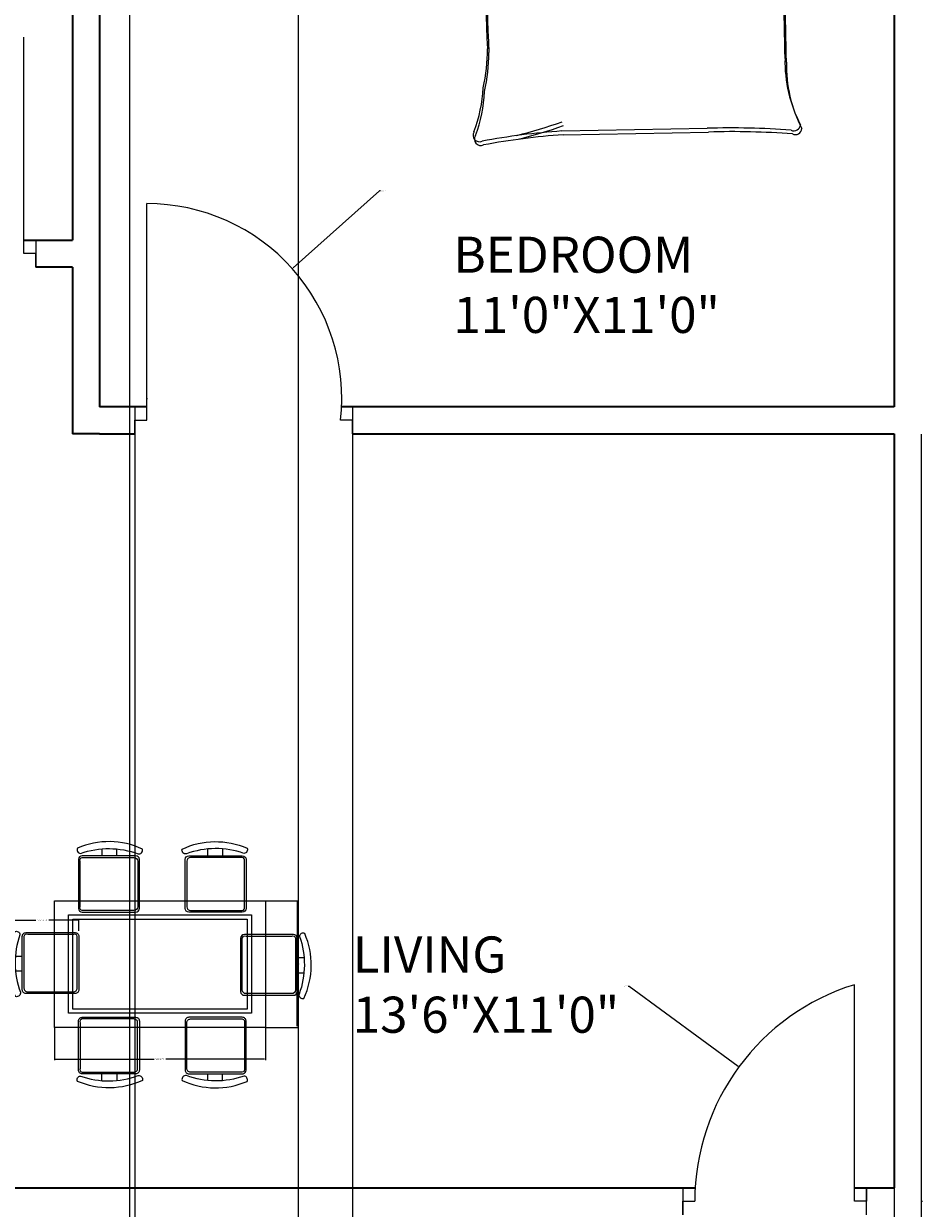
# Model space of a CAD drawing. Units: inches. Extents: x 1721 to 2510, y 1544 to 2360.
# Tile 7 of 10: x 1940 to 2090, y 1988 to 2185. Entities that reach past the tile are written whole.
import ezdxf

# ---------------------------------------------------------------- set-up
doc = ezdxf.new("R2010")
doc.units = ezdxf.units.IN
for name, color, linetype, lineweight in [('A-ANNO-DIMS', 2, 'Continuous', 18), ('A-AREA-IDEN', 7, 'Continuous', 18), ('A-DOOR', 3, 'Continuous', 18), ('A-FURN', 8, 'Continuous', 13), ('A-WALL', 7, 'Continuous', 35)]:
    doc.layers.add(name, color=color, linetype=linetype, lineweight=lineweight)
doc.styles.get("Standard").update_dxf_attribs({"font": 'arial.ttf'})
doc.dimstyles.get("Standard").update_dxf_attribs({"dimtxt": 0.18, "dimasz": 0.18, "dimexe": 0.18, "dimexo": 0.0625, "dimgap": 0.09, "dimtad": 0, "dimtih": 1, "dimtoh": 1, "dimdec": 4, "dimzin": 0, "dimdsep": 46, "dimtxsty": 'Standard', "dimcen": 0.09, "dimadec": 0, "dimazin": 0, "dimtfac": 1, "dimtdec": 4, "dimtofl": 0, "dimtmove": 0, "dimatfit": 3, "dimfxl": 1, "dimtolj": 1, "dimtzin": 0, "dimarcsym": 0})

# ---------------------------------------------------------------- blocks, each defined once
blk = doc.blocks.new('BED-DOUBLE')
for p, q in [((39.64, 78.43), (15.52, 78.72)), ((39.64, 78.43), (15.52, 78.72)), ((39.86, 77.8), (15.74, 78.09)), ((39.86, 77.8), (15.74, 78.09)), ((1.93, 30.11), (1.99, 28.4, 3.79)), ((1.93, 30.11), (1.99, 28.4, 3.79)), ((15.66, 30.21), (13.68, 29.32)), ((15.66, 30.21), (13.68, 29.32)), ((15.88, 29.58), (13.89, 28.69)), ((15.88, 29.58), (13.89, 28.69)), ((18.1, 30.79), (15.66, 30.21)), ((18.1, 30.79), (15.66, 30.21)), ((18.31, 30.16), (15.88, 29.58)), ((18.31, 30.16), (15.88, 29.58)), ((18.38, 28.81), (18.1, 30.79)), ((18.38, 28.81), (18.1, 30.79)), ((18.59, 28.18), (18.31, 30.16)), ((18.59, 28.18), (18.31, 30.16)), ((3.5, 28.99), (1.99, 28.4)), ((3.5, 28.99), (1.99, 28.4)), ((1.99, 28.4), (5.58, 25.17)), ((1.99, 28.4), (5.58, 25.17)), ((2.15, 29.48), (2.21, 27.77, 3.79)), ((2.15, 29.48), (2.21, 27.77, 3.79)), ((3.72, 28.36), (2.21, 27.77)), ((3.72, 28.36), (2.21, 27.77)), ((2.21, 27.77), (5.8, 24.54)), ((2.21, 27.77), (5.8, 24.54)), ((6.54, 28.65), (3.5, 28.99)), ((6.54, 28.65), (3.5, 28.99)), ((6.75, 28.02), (3.72, 28.36)), ((6.75, 28.02), (3.72, 28.36)), ((10.33, 28.91), (6.54, 28.65)), ((10.33, 28.91), (6.54, 28.65)), ((10.55, 28.28), (6.75, 28.02)), ((10.55, 28.28), (6.75, 28.02)), ((13.68, 29.32), (10.33, 28.91)), ((13.68, 29.32), (10.33, 28.91)), ((13.89, 28.69), (10.55, 28.28)), ((13.89, 28.69), (10.55, 28.28)), ((20, 24.39), (18.38, 28.81)), ((20, 24.39), (18.38, 28.81)), ((20.21, 23.76), (18.59, 28.18)), ((20.21, 23.76), (18.59, 28.18)), ((3.23, 1.19), (3.55, 27.27)), ((3.23, 1.19), (3.55, 27.27)), ((3.45, 0.56), (3.76, 26.64)), ((3.45, 0.56), (3.76, 26.64)), ((5.58, 25.17), (8.44, 23.01)), ((5.58, 25.17), (8.44, 23.01)), ((5.8, 24.54), (8.66, 22.38)), ((5.8, 24.54), (8.66, 22.38)), ((24.03, 17.98), (20, 24.39)), ((24.03, 17.98), (20, 24.39)), ((24.24, 17.35), (20.21, 23.76)), ((24.24, 17.35), (20.21, 23.76)), ((8.44, 23.01), (13.88, 20.98)), ((8.44, 23.01), (13.88, 20.98)), ((8.66, 22.38), (14.1, 20.35)), ((8.66, 22.38), (14.1, 20.35)), ((13.88, 20.98), (22.02, 18)), ((13.88, 20.98), (22.02, 18)), ((14.1, 20.35), (22.24, 17.37)), ((14.1, 20.35), (22.24, 17.37)), ((50.28, 18.38), (50.07, 0.63)), ((50.28, 18.38), (50.07, 0.63)), ((50.5, 17.75), (50.29, 0)), ((50.5, 17.75), (50.29, 0)), ((9.01, 16.97), (3.98, 17.42)), ((3.98, 17.42), (4.71, 14.34)), ((9.01, 16.97), (3.98, 17.42)), ((3.98, 17.42), (4.71, 14.34)), ((9.23, 16.34), (4.2, 16.8)), ((4.2, 16.8), (4.92, 13.71)), ((9.23, 16.34), (4.2, 16.8)), ((4.2, 16.8), (4.92, 13.71)), ((10.94, 17.49), (9.01, 16.97)), ((10.94, 17.49), (9.01, 16.97)), ((11.15, 16.86), (9.23, 16.34)), ((11.15, 16.86), (9.23, 16.34)), ((17.8, 16.99), (10.94, 17.49)), ((17.8, 16.99), (10.94, 17.49)), ((18.02, 16.36), (11.15, 16.86)), ((18.02, 16.36), (11.15, 16.86)), ((21.75, 16.29), (17.8, 16.99)), ((21.75, 16.29), (17.8, 16.99)), ((21.96, 15.66), (18.02, 16.36)), ((21.96, 15.66), (18.02, 16.36)), ((23.54, 17.35), (20.51, 16.13)), ((23.54, 17.35), (20.51, 16.13)), ((23.75, 16.73), (20.73, 15.5)), ((23.75, 16.73), (20.73, 15.5)), ((25.94, 17.48), (23.54, 17.35)), ((25.94, 17.48), (23.54, 17.35)), ((26.16, 16.85), (23.75, 16.73)), ((26.16, 16.85), (23.75, 16.73)), ((26.07, 14.85), (25.94, 17.48)), ((26.07, 14.85), (25.94, 17.48)), ((26.29, 14.22), (26.16, 16.85)), ((26.29, 14.22), (26.16, 16.85)), ((27.61, 14.21), (27.64, 16.84)), ((27.61, 14.21), (27.64, 16.84)), ((27.64, 16.84), (30.05, 16.81)), ((27.64, 16.84), (30.05, 16.81)), ((27.82, 13.58), (27.85, 16.21)), ((27.82, 13.58), (27.85, 16.21)), ((27.85, 16.21), (30.26, 16.18)), ((27.85, 16.21), (30.26, 16.18)), ((34.67, 16.66), (29.65, 17.12)), ((34.67, 16.66), (29.65, 17.12)), ((34.89, 16.03), (29.86, 16.49)), ((34.89, 16.03), (29.86, 16.49)), ((30.05, 16.81), (33.11, 15.7)), ((30.05, 16.81), (33.11, 15.7)), ((30.26, 16.18), (33.33, 15.07)), ((30.26, 16.18), (33.33, 15.07)), ((36.6, 17.19), (34.67, 16.66)), ((36.6, 17.19), (34.67, 16.66)), ((36.81, 16.56), (34.89, 16.03)), ((36.81, 16.56), (34.89, 16.03)), ((43.46, 16.68), (36.6, 17.19)), ((43.46, 16.68), (36.6, 17.19)), ((43.68, 16.05), (36.81, 16.56)), ((43.68, 16.05), (36.81, 16.56)), ((43.46, 16.68), (44.58, 16.98)), ((43.46, 16.68), (44.58, 16.98)), ((47.41, 15.98), (43.46, 16.68)), ((47.41, 15.98), (43.46, 16.68)), ((43.68, 16.05), (44.79, 16.35)), ((43.68, 16.05), (44.79, 16.35)), ((47.62, 15.35), (43.68, 16.05)), ((47.62, 15.35), (43.68, 16.05)), ((44.58, 16.98), (49.58, 17.63)), ((44.58, 16.98), (49.58, 17.63)), ((44.79, 16.35), (49.8, 17)), ((44.79, 16.35), (49.8, 17)), ((49.58, 17.63), (48.98, 14.52)), ((49.58, 17.63), (48.98, 14.52)), ((49.8, 17), (49.19, 13.89)), ((49.8, 17), (49.19, 13.89)), ((4.71, 14.34), (4.5, 12.77)), ((4.71, 14.34), (4.5, 12.77)), ((26.73, 13.04), (26.07, 14.85)), ((26.73, 13.04), (26.07, 14.85)), ((26.95, 12.41), (26.29, 14.22)), ((26.95, 12.41), (26.29, 14.22)), ((27.02, 12.38), (27.61, 14.21)), ((27.02, 12.38), (27.61, 14.21)), ((48.98, 14.52), (49.24, 12.96)), ((48.98, 14.52), (49.24, 12.96)), ((49.19, 13.89), (49.46, 12.33)), ((49.19, 13.89), (49.46, 12.33)), ((4.5, 12.77), (5.25, 9.26)), ((4.5, 12.77), (5.25, 9.26)), ((4.92, 13.71), (4.72, 12.14)), ((4.92, 13.71), (4.72, 12.14)), ((4.72, 12.14), (5.46, 8.63)), ((4.72, 12.14), (5.46, 8.63)), ((26.8, 11.77), (26.73, 13.04)), ((26.8, 11.77), (26.73, 13.04)), ((27.01, 11.14), (26.95, 12.41)), ((27.01, 11.14), (26.95, 12.41)), ((27, 11.1), (27.02, 12.38)), ((27, 11.1), (27.02, 12.38)), ((27.23, 11.75), (27.82, 13.58)), ((27.23, 11.75), (27.82, 13.58)), ((49.24, 12.96), (48.63, 9.42)), ((49.24, 12.96), (48.63, 9.42)), ((49.46, 12.33), (48.85, 8.79)), ((49.46, 12.33), (48.85, 8.79)), ((4.25, 9.35), (4.77, 10.37)), ((4.25, 9.35), (4.77, 10.37)), ((26.39, 8.62), (26.8, 11.77)), ((26.39, 8.62), (26.8, 11.77)), ((26.61, 7.99), (27.01, 11.14)), ((26.61, 7.99), (27.01, 11.14)), ((27.53, 7.98), (27, 11.1)), ((27.53, 7.98), (27, 11.1)), ((27.22, 10.47), (27.23, 11.75)), ((27.22, 10.47), (27.23, 11.75)), ((27.75, 7.35), (27.22, 10.47)), ((27.75, 7.35), (27.22, 10.47)), ((49.63, 9.55), (49.07, 10.55)), ((49.63, 9.55), (49.07, 10.55)), ((49.84, 8.92), (49.29, 9.92)), ((49.84, 8.92), (49.29, 9.92)), ((4.8, 6.82), (4.25, 9.35)), ((4.8, 6.82), (4.25, 9.35)), ((4.47, 8.72), (4.98, 9.74)), ((4.47, 8.72), (4.98, 9.74)), ((5.02, 6.19), (4.47, 8.72)), ((5.02, 6.19), (4.47, 8.72)), ((5.25, 9.26), (6.37, 6.62)), ((5.25, 9.26), (6.37, 6.62)), ((5.46, 8.63), (6.59, 5.99)), ((5.46, 8.63), (6.59, 5.99)), ((26.09, 3.36), (26.39, 8.62)), ((26.09, 3.36), (26.39, 8.62)), ((26.3, 2.73), (26.61, 7.99)), ((26.3, 2.73), (26.61, 7.99)), ((28.04, 2.73), (27.53, 7.98)), ((28.04, 2.73), (27.53, 7.98)), ((48.63, 9.42), (47.61, 6.74)), ((48.63, 9.42), (47.61, 6.74)), ((48.85, 8.79), (47.82, 6.11)), ((48.85, 8.79), (47.82, 6.11)), ((49.17, 7.01), (49.63, 9.55)), ((49.17, 7.01), (49.63, 9.55)), ((49.39, 6.38), (49.84, 8.92)), ((49.39, 6.38), (49.84, 8.92)), ((4.39, 3.68), (4.8, 6.82)), ((4.39, 3.68), (4.8, 6.82)), ((4.61, 3.05), (5.02, 6.19)), ((4.61, 3.05), (5.02, 6.19)), ((28.25, 2.1), (27.75, 7.35)), ((28.25, 2.1), (27.75, 7.35)), ((49.7, 3.88), (49.17, 7.01)), ((49.7, 3.88), (49.17, 7.01)), ((49.92, 3.25), (49.39, 6.38)), ((49.92, 3.25), (49.39, 6.38)), ((8.71, 3.62), (12.44, 4.09)), ((8.71, 3.62), (12.44, 4.09)), ((12.44, 4.09), (17.76, 5.35)), ((12.44, 4.09), (17.76, 5.35)), ((12.65, 3.46), (17.98, 4.72)), ((12.65, 3.46), (17.98, 4.72)), ((15.1, 4.65), (17.12, 4.04)), ((15.1, 4.65), (17.12, 4.04)), ((15.32, 4.02), (17.34, 3.41)), ((15.32, 4.02), (17.34, 3.41)), ((17.12, 4.04), (19.98, 3.48)), ((17.12, 4.04), (19.98, 3.48)), ((41.65, 3.98), (36.28, 5.04)), ((41.65, 3.98), (36.28, 5.04)), ((41.87, 3.35), (36.49, 4.41)), ((41.87, 3.35), (36.49, 4.41)), ((38.96, 4.44), (36.97, 3.75)), ((38.96, 4.44), (36.97, 3.75)), ((45.39, 3.65), (41.65, 3.98)), ((45.39, 3.65), (41.65, 3.98)), ((50.09, 2.13), (3.25, 2.69)), ((50.09, 2.13), (3.25, 2.69)), ((50.31, 1.5), (3.47, 2.06)), ((50.31, 1.5), (3.47, 2.06)), ((4.39, 3.68), (9.69, 3.52)), ((4.39, 3.68), (9.69, 3.52)), ((4.61, 3.05), (9.9, 2.89)), ((4.61, 3.05), (9.9, 2.89)), ((9.69, 3.52), (8.71, 3.62)), ((9.69, 3.52), (8.71, 3.62)), ((8.92, 2.99), (12.65, 3.46)), ((8.92, 2.99), (12.65, 3.46)), ((9.9, 2.89), (8.92, 2.99)), ((9.9, 2.89), (8.92, 2.99)), ((17.34, 3.41), (20.2, 2.85)), ((17.34, 3.41), (20.2, 2.85)), ((19.98, 3.48), (20.3, 3.49)), ((19.98, 3.48), (20.3, 3.49)), ((20.2, 2.85), (20.52, 2.86)), ((20.2, 2.85), (20.52, 2.86)), ((20.3, 3.49), (24.64, 3.85)), ((20.3, 3.49), (24.64, 3.85)), ((20.52, 2.86), (24.86, 3.22)), ((20.52, 2.86), (24.86, 3.22)), ((24.64, 3.85), (26.09, 3.36)), ((24.64, 3.85), (26.09, 3.36)), ((24.86, 3.22), (26.3, 2.73)), ((24.86, 3.22), (26.3, 2.73)), ((29.46, 3.28), (28.04, 2.73)), ((29.46, 3.28), (28.04, 2.73)), ((29.68, 2.65), (28.25, 2.1)), ((29.68, 2.65), (28.25, 2.1)), ((33.81, 3.08), (29.46, 3.28)), ((33.81, 3.08), (29.46, 3.28)), ((34.03, 2.45), (29.68, 2.65)), ((34.03, 2.45), (29.68, 2.65)), ((34.13, 3.08), (33.81, 3.08)), ((34.13, 3.08), (33.81, 3.08)), ((34.35, 2.45), (34.03, 2.45)), ((34.35, 2.45), (34.03, 2.45)), ((36.97, 3.75), (34.13, 3.08)), ((36.97, 3.75), (34.13, 3.08)), ((37.19, 3.12), (34.35, 2.45)), ((37.19, 3.12), (34.35, 2.45)), ((39.18, 3.81), (37.19, 3.12)), ((39.18, 3.81), (37.19, 3.12)), ((45.61, 3.02), (41.87, 3.35)), ((45.61, 3.02), (41.87, 3.35)), ((45.5, 3.63), (45.39, 3.65)), ((45.5, 3.63), (45.39, 3.65)), ((49.7, 3.91), (45.5, 3.63)), ((49.7, 3.91), (45.5, 3.63)), ((45.71, 3), (45.61, 3.02)), ((45.71, 3), (45.61, 3.02)), ((49.91, 3.28), (45.71, 3)), ((49.91, 3.28), (45.71, 3)), ((50.07, 0.63), (3.23, 1.19)), ((50.07, 0.63), (3.23, 1.19)), ((50.29, 0), (3.45, 0.56)), ((50.29, 0), (3.45, 0.56))]:
    blk.add_line(p, q)
for centre, radius, start, end in [((1.08, 78.52), 1.08, 61.9736, 175.3348), ((1.08, 78.52), 1.08, 61.9736, 175.3348), ((1.29, 77.89), 1.08, 61.9736, 175.3348), ((1.29, 77.89), 1.08, 61.9736, 175.3348), ((15.63, 209.12), 130.4, 263.8146, 269.9499), ((15.63, 209.12), 130.4, 263.8146, 269.9499), ((15.85, 208.49), 130.4, 263.8146, 269.9499), ((15.85, 208.49), 130.4, 263.8146, 269.9499), ((70.08, -22.85), 104.34, 102.698, 107.0202), ((70.08, -22.85), 104.34, 102.698, 107.0202), ((34.83, 197.67), 119.34, 272.3106, 278.7239), ((34.83, 197.67), 119.34, 272.3106, 278.7239), ((35.05, 197.04), 119.34, 272.3106, 278.7239), ((35.05, 197.04), 119.34, 272.3106, 278.7239), ((53.35, 78.73), 1.07, 325.4884, 112.793), ((53.35, 78.73), 1.07, 325.4884, 112.793), ((53.56, 78.1), 1.07, 325.4884, 112.793), ((53.56, 78.1), 1.07, 325.4884, 112.793), ((-20.36, 68.78), 22.61, 356.7862, 25.7829), ((-20.36, 68.78), 22.61, 356.7862, 25.7829), ((-20.14, 68.15), 22.61, 356.7862, 25.7829), ((-20.14, 68.15), 22.61, 356.7862, 25.7829), ((70.29, -23.48), 104.34, 102.698, 107.0202), ((70.29, -23.48), 104.34, 102.698, 107.0202), ((75.53, 69.21), 23.09, 157.2899, 175.9668), ((75.53, 69.21), 23.09, 157.2899, 175.9668), ((75.75, 68.58), 23.09, 157.2899, 175.9668), ((75.75, 68.58), 23.09, 157.2899, 175.9668), ((80.6, 63.5), 29.05, 165.3797, 178.2261), ((80.6, 63.5), 29.05, 165.3797, 178.2261), ((80.81, 62.87), 29.05, 165.3797, 178.2261), ((80.81, 62.87), 29.05, 165.3797, 178.2261), ((4473.12, 14.21), 4471.22, 179.317, 179.60172), ((4473.12, 14.21), 4471.22, 179.317, 179.60172), ((4473.34, 13.58), 4471.22, 179.317, 179.60172), ((4473.34, 13.58), 4471.22, 179.317, 179.60172), ((-421.08, 55.88), 472.73, 357.5425, 1.0334), ((-421.08, 55.88), 472.73, 357.5425, 1.0334), ((-420.87, 55.25), 472.73, 357.5425, 1.0334), ((-420.87, 55.25), 472.73, 357.5425, 1.0334), ((-124.73, 38.32), 126.93, 356.294, 3.1513), ((-124.73, 38.32), 126.93, 356.294, 3.1513), ((-124.51, 37.69), 126.93, 356.294, 3.1513), ((-124.51, 37.69), 126.93, 356.294, 3.1513), ((217.81, 29.18), 166.73, 177.791, 180.323), ((217.81, 29.18), 166.73, 177.791, 180.323), ((218.03, 28.55), 166.73, 177.791, 180.323), ((218.03, 28.55), 166.73, 177.791, 180.323), ((3.1, -5.33), 35.46, 79.1911, 91.8805), ((3.1, -5.33), 35.46, 79.1911, 91.8805), ((11.02, 35.47), 6.1, 257.9756, 293.0532), ((11.02, 35.47), 6.1, 257.9756, 293.0532), ((22.96, 2.41), 29.06, 99.9765, 109.1954), ((22.96, 2.41), 29.06, 99.9765, 109.1954), ((23.18, 1.78), 29.06, 99.9765, 109.1954), ((23.18, 1.78), 29.06, 99.9765, 109.1954), ((17.93, 30.85), 0.181, 339.5612, 90.4525), ((17.93, 30.85), 0.181, 339.5612, 90.4525), ((18.15, 30.22), 0.181, 339.5612, 90.4525), ((18.15, 30.22), 0.181, 339.5612, 90.4525), ((3.31, -5.96), 35.46, 79.1911, 91.8805), ((3.31, -5.96), 35.46, 79.1911, 91.8805), ((11.23, 34.84), 6.1, 257.9756, 293.0532), ((11.23, 34.84), 6.1, 257.9756, 293.0532), ((37.91, 154), 126.46, 261.0993, 276.2154), ((37.91, 154), 126.46, 261.0993, 276.2154), ((38.12, 153.37), 126.46, 261.0993, 276.2154), ((38.12, 153.37), 126.46, 261.0993, 276.2154), ((-29.75, 21.28), 81.65, 358.0366, 4.9188), ((-29.75, 21.28), 81.65, 358.0366, 4.9188), ((-29.53, 20.65), 81.65, 358.0366, 4.9188), ((-29.53, 20.65), 81.65, 358.0366, 4.9188), ((34.68, 179.26), 161.69, 265.4014, 276.097), ((34.68, 179.26), 161.69, 265.4014, 276.097), ((34.89, 178.63), 161.69, 265.4014, 276.097), ((34.89, 178.63), 161.69, 265.4014, 276.097)]:
    blk.add_arc(centre, radius, start, end)
blk = doc.blocks.new('TABLE-DINING-RECT')
for points in [[(0, 21.04), (35.07, 21.04), (35.07, 0), (0, 0)], [(2.34, 18.71), (32.73, 18.71), (32.73, 2.34), (2.34, 2.34)], [(3.04, 18), (32.03, 18), (32.03, 3.04), (3.04, 3.04)]]:
    blk.add_lwpolyline(points, close=True)
blk = doc.blocks.new('CHAIR-DINING-A')
for points in [[(2.02, 0.75, -0.578392), (1.23, 0.03, -0.214524), (1.08, 10.81, -0.552014), (1.95, 10.31, 0.175809), (2.02, 0.75)], [(2.34, 10.03, -0.414214), (2.96, 10.65), (11.11, 10.65, -0.414214), (11.73, 10.03), (11.73, 1.16, -0.414214), (11.11, 0.54), (2.96, 0.54, -0.414214), (2.34, 1.16), (2.34, 10.03)], [(2.34, 4.27), (1.21, 4.27, 0.064759)]]:
    blk.add_lwpolyline(points, format="xyb")
blk.add_lwpolyline([(2.62, 10.02), (2.62, 1.44, 0.414214), (3.24, 0.82), (10.83, 0.82, 0.414214), (11.45, 1.44), (11.45, 10.02, 0.512069), (10.83, 10.37), (3.24, 10.37, 0.512069)], format="xyb", close=True)
blk.add_lwpolyline([(1.19, 6.76), (2.34, 6.76)])
blk = doc.blocks.new('CHAIR-DINING-B')
for points in [[(9.72, 2.34), (0.85, 2.34, -0.414214), (0.23, 2.96), (0.23, 11.11, -0.414214), (0.85, 11.73), (9.72, 11.73, -0.414214), (10.34, 11.11), (10.34, 2.96, -0.414214), (9.72, 2.34)], [(10.13, 2.03, -0.578392), (10.85, 1.23, -0.214524), (0.07, 1.08, -0.552014), (0.57, 1.95, 0.175809), (10.13, 2.03)], [(6.61, 2.34), (6.61, 1.21, 0.064759)]]:
    blk.add_lwpolyline(points, format="xyb")
blk.add_lwpolyline([(0.86, 2.62), (9.44, 2.62, 0.414214), (10.06, 3.24), (10.06, 10.83, 0.414214), (9.44, 11.45), (0.86, 11.45, 0.512069), (0.51, 10.83), (0.51, 3.24, 0.512069)], format="xyb", close=True)
blk.add_lwpolyline([(4.12, 1.19), (4.12, 2.34)])
blk = doc.blocks.new('CHAIR-DINING-C')
for points in [[(10.03, 2.34, 0.414214), (10.65, 2.96), (10.65, 11.11, 0.414214), (10.03, 11.73), (1.16, 11.73, 0.414214), (0.54, 11.11), (0.54, 2.96, 0.414214), (1.16, 2.34), (10.03, 2.34)], [(10.31, 1.95, -0.175809), (0.75, 2.03, 0.578392), (0.03, 1.23, 0.214524), (10.81, 1.08, 0.552014), (10.31, 1.95, -0.065079)], [(4.27, 2.34), (4.27, 1.21, -0.064759)]]:
    blk.add_lwpolyline(points, format="xyb")
blk.add_lwpolyline([(10.02, 2.62), (1.44, 2.62, -0.414214), (0.82, 3.24), (0.82, 10.83, -0.414214), (1.44, 11.45), (10.02, 11.45, -0.512069), (10.37, 10.83), (10.37, 3.24, -0.512069)], format="xyb", close=True)
blk.add_lwpolyline([(6.76, 1.19), (6.76, 2.34)])
blk = doc.blocks.new('*D16')
at = {"layer": 'A-ANNO-DIMS', "color": 0, "lineweight": -2, "transparency": 16777216}
for p, q in [((1945.52, 2017.72), (1945.52, 2012.34)), ((1980.6, 2017.72), (1980.6, 2012.34)), ((1945.7, 2012.52), (1962.1, 2012.52)), ((1980.42, 2012.52), (1964.02, 2012.52))]:
    blk.add_line(p, q, dxfattribs=at)
at = {"layer": 'A-ANNO-DIMS', "color": 0, "transparency": 16777216}
for points in [[(1945.7, 2012.55), (1945.7, 2012.49), (1945.52, 2012.52)], [(1980.42, 2012.55), (1980.42, 2012.49), (1980.6, 2012.52)]]:
    blk.add_solid(points, dxfattribs=at)
at = {"layer": 'Defpoints', "color": 0, "transparency": 16777216}
for p in [(1945.52, 2017.78), (1980.6, 2017.78), (1980.6, 2012.52)]:
    blk.add_point(p, dxfattribs=at)
at = {"layer": 'A-ANNO-DIMS', "color": 0, "transparency": 16777216, "insert": (1963.06, 2012.52), "char_height": 0.18, "attachment_point": 5}
blk.add_mtext('\\A1;TABLE 35 TYP.', dxfattribs=at)
blk = doc.blocks.new('*D17')
at = {"layer": 'A-ANNO-DIMS', "color": 0, "lineweight": -2, "transparency": 16777216}
for p, q in [((1980.66, 2038.82), (1986.04, 2038.82)), ((1985.86, 2038.64), (1985.86, 2028.48)), ((1985.86, 2017.96), (1985.86, 2028.12)), ((1980.66, 2017.78), (1986.04, 2017.78))]:
    blk.add_line(p, q, dxfattribs=at)
at = {"layer": 'A-ANNO-DIMS', "color": 0, "transparency": 16777216}
for points in [[(1985.83, 2038.64), (1985.89, 2038.64), (1985.86, 2038.82)], [(1985.83, 2017.96), (1985.89, 2017.96), (1985.86, 2017.78)]]:
    blk.add_solid(points, dxfattribs=at)
at = {"layer": 'Defpoints', "color": 0, "transparency": 16777216}
for p in [(1980.6, 2038.82), (1985.86, 2038.82), (1980.6, 2017.78)]:
    blk.add_point(p, dxfattribs=at)
at = {"layer": 'A-ANNO-DIMS', "color": 0, "transparency": 16777216, "insert": (1985.86, 2028.3), "char_height": 0.18, "attachment_point": 5}
blk.add_mtext('\\A1;21 TYP.', dxfattribs=at)
blk = doc.blocks.new('*D30')
at = {"layer": 'A-ANNO-DIMS', "color": 0, "lineweight": -2, "transparency": 16777216}
for p, q in [((1937.43, 2033.84), (1937.43, 2035.78)), ((1937.61, 2035.6), (1942.43, 2035.6)), ((1949.39, 2035.6), (1944.57, 2035.6)), ((1949.57, 2033.84), (1949.57, 2035.78))]:
    blk.add_line(p, q, dxfattribs=at)
at = {"layer": 'A-ANNO-DIMS', "color": 0, "transparency": 16777216}
for points in [[(1937.61, 2035.63), (1937.61, 2035.57), (1937.43, 2035.6)], [(1949.39, 2035.63), (1949.39, 2035.57), (1949.57, 2035.6)]]:
    blk.add_solid(points, dxfattribs=at)
at = {"layer": 'Defpoints', "color": 0, "transparency": 16777216}
for p in [(1949.57, 2035.6), (1937.43, 2033.78), (1949.57, 2033.78)]:
    blk.add_point(p, dxfattribs=at)
at = {"layer": 'A-ANNO-DIMS', "color": 0, "transparency": 16777216, "insert": (1943.5, 2035.6), "char_height": 0.18, "attachment_point": 5}
blk.add_mtext('\\A1;CHAIR A 12 TYP.', dxfattribs=at)
blk = doc.blocks.new('*D62')
at = {"layer": 'A-ANNO-DIMS', "color": 0, "lineweight": -2, "transparency": 16777216}
for p, q in [((1957.99, 2252.88), (1957.99, 1606.75)), ((1986.02, 2252.88), (1986.02, 1606.75)), ((1958.17, 1606.93), (1971.61, 1606.93)), ((1985.84, 1606.93), (1972.4, 1606.93))]:
    blk.add_line(p, q, dxfattribs=at)
at = {"layer": 'A-ANNO-DIMS', "color": 0, "transparency": 16777216}
for points in [[(1958.17, 1606.96), (1958.17, 1606.9), (1957.99, 1606.93)], [(1985.84, 1606.96), (1985.84, 1606.9), (1986.02, 1606.93)]]:
    blk.add_solid(points, dxfattribs=at)
at = {"layer": 'Defpoints', "color": 0, "transparency": 16777216}
for p in [(1957.99, 2252.94), (1986.02, 2252.94), (1986.02, 1606.93)]:
    blk.add_point(p, dxfattribs=at)
at = {"layer": 'A-ANNO-DIMS', "color": 0, "transparency": 16777216, "insert": (1972.01, 1606.93), "char_height": 0.18, "attachment_point": 5}
blk.add_mtext('\\A1;28.03', dxfattribs=at)
blk = doc.blocks.new('*D63')
at = {"layer": 'A-ANNO-DIMS', "color": 0, "lineweight": -2, "transparency": 16777216}
for p, q in [((1958.89, 2116.38), (1958.89, 1606.75)), ((1995.05, 2116.38), (1995.05, 1606.75)), ((1959.07, 1606.93), (1976.58, 1606.93)), ((1994.87, 1606.93), (1977.36, 1606.93))]:
    blk.add_line(p, q, dxfattribs=at)
at = {"layer": 'A-ANNO-DIMS', "color": 0, "transparency": 16777216}
for points in [[(1959.07, 1606.96), (1959.07, 1606.9), (1958.89, 1606.93)], [(1994.87, 1606.96), (1994.87, 1606.9), (1995.05, 1606.93)]]:
    blk.add_solid(points, dxfattribs=at)
at = {"layer": 'Defpoints', "color": 0, "transparency": 16777216}
for p in [(1958.89, 2116.44), (1995.05, 2116.44), (1995.05, 1606.93)]:
    blk.add_point(p, dxfattribs=at)
at = {"layer": 'A-ANNO-DIMS', "color": 0, "transparency": 16777216, "insert": (1976.97, 1606.93), "char_height": 0.18, "attachment_point": 5}
blk.add_mtext('\\A1;36.16', dxfattribs=at)
blk = doc.blocks.new('*D65')
at = {"layer": 'A-ANNO-DIMS', "color": 0, "lineweight": -2, "transparency": 16777216}
for p, q in [((2085, 2116.38), (2085, 1606.75)), ((2089.5, 2116.38), (2089.5, 1606.75)), ((2085.18, 1606.93), (2086.99, 1606.93)), ((2089.32, 1606.93), (2087.51, 1606.93))]:
    blk.add_line(p, q, dxfattribs=at)
at = {"layer": 'A-ANNO-DIMS', "color": 0, "transparency": 16777216}
for points in [[(2085.18, 1606.96), (2085.18, 1606.9), (2085, 1606.93)], [(2089.32, 1606.96), (2089.32, 1606.9), (2089.5, 1606.93)]]:
    blk.add_solid(points, dxfattribs=at)
at = {"layer": 'Defpoints', "color": 0, "transparency": 16777216}
for p in [(2085, 2116.44), (2089.5, 2116.44), (2089.5, 1606.93)]:
    blk.add_point(p, dxfattribs=at)
at = {"layer": 'A-ANNO-DIMS', "color": 0, "transparency": 16777216, "insert": (2087.25, 1606.93), "char_height": 0.18, "attachment_point": 5}
blk.add_mtext('\\A1;4.5', dxfattribs=at)
blk = doc.blocks.new('*D68')
at = {"layer": 'A-ANNO-DIMS', "color": 0, "lineweight": -2, "transparency": 16777216}
for p, q in [((2040.83, 2024.64), (2041.01, 2024.64)), ((2041.01, 2024.64), (2059.08, 2011.34)), ((2089.5, 1988.88), (2089.68, 1988.88)), ((2089.59, 1988.79), (2089.59, 1988.97))]:
    blk.add_line(p, q, dxfattribs=at)
at = {"layer": 'A-ANNO-DIMS', "color": 0, "transparency": 16777216}
blk.add_solid([(2059.1, 2011.36), (2059.06, 2011.31), (2059.23, 2011.23)], dxfattribs=at)
at = {"layer": 'Defpoints', "color": 0, "transparency": 16777216}
for p in [(2059.23, 2011.23), (2089.59, 1988.88)]:
    blk.add_point(p, dxfattribs=at)
at = {"layer": 'A-ANNO-DIMS', "color": 0, "transparency": 16777216, "insert": (2040.42, 2024.64), "char_height": 0.18, "attachment_point": 5}
blk.add_mtext('\\A1;R37.7', dxfattribs=at)
blk = doc.blocks.new('*D74')
at = {"layer": 'A-ANNO-DIMS', "color": 0, "lineweight": -2, "transparency": 16777216}
for p, q in [((1999.51, 2156.83), (1985.16, 2144.01)), ((1999.69, 2156.83), (1999.51, 2156.83)), ((1960.8, 2122.32), (1960.98, 2122.32)), ((1960.89, 2122.23), (1960.89, 2122.41))]:
    blk.add_line(p, q, dxfattribs=at)
at = {"layer": 'A-ANNO-DIMS', "color": 0, "transparency": 16777216}
blk.add_solid([(1985.14, 2144.03), (1985.18, 2143.99), (1985.03, 2143.89)], dxfattribs=at)
at = {"layer": 'Defpoints', "color": 0, "transparency": 16777216}
for p in [(1985.03, 2143.89), (1960.89, 2122.32)]:
    blk.add_point(p, dxfattribs=at)
at = {"layer": 'A-ANNO-DIMS', "color": 0, "transparency": 16777216, "insert": (2000.17, 2156.83), "char_height": 0.18, "attachment_point": 5}
blk.add_mtext('\\A1;R32.37', dxfattribs=at)

msp = doc.modelspace()

# ---------------------------------------------------------------- linework, layer by layer
at = {"layer": 'A-DOOR'}
for p, q in [((1940.4212, 2146.3798), (1940.4212, 2182.3798)), ((1960.8889, 2118.6915), (1960.8889, 2154.6915)), ((1942.4212, 2148.6298), (1942.4212, 2144.1298)), ((1942.4212, 2146.3798), (1940.4212, 2146.3798)), ((1942.4212, 2144.1298), (1942.4212, 2146.3798)), ((1958.8889, 2120.9415), (1958.8889, 2116.4415)), ((1995.0512, 2120.9415), (1995.0512, 2116.4415)), ((1958.8889, 2116.4415), (1958.8889, 2118.6915)), ((1958.8889, 2118.6915), (1958.8889, 2118.6915)), ((1958.8889, 2118.6915), (1960.8889, 2118.6915)), ((1995.0512, 2118.6915), (1993.0512, 2118.6915)), ((1995.0512, 2116.4415), (1995.0512, 2118.6915)), ((2078.3854, 1988.8798), (2078.3854, 2024.8798)), ((2049.8856, 1991.1298), (2049.8856, 1986.6298)), ((2080.3854, 1986.6298), (2080.3854, 1991.1298)), ((2080.3854, 1991.1298), (2080.3854, 1988.8798)), ((2049.8856, 1986.6298), (2049.8856, 1988.8798)), ((2049.8856, 1988.8798), (2051.8856, 1988.8798)), ((2080.3854, 1988.8798), (2078.3854, 1988.8798))]:
    msp.add_line(p, q, dxfattribs=at)
for centre, radius, start, end in [((1960.8889, 2122.3247), 32.3669, 353.555037, 90), ((2089.5886, 1988.8798), 37.7029, 107.286074, 180)]:
    msp.add_arc(centre, radius, start, end, dxfattribs=at)
at = {"layer": 'A-FURN'}
for points in [[(1949.8609, 2046.6962, -0.17580919), (1959.4137, 2046.6239, 0.57839206), (1960.1374, 2047.4196, 0.21452438), (1949.3543, 2047.5643, 0.55201397), (1949.8609, 2046.6962, -0.06507904)], [(1967.456, 2046.6239, -0.57839206), (1966.7323, 2047.4196, -0.21452438), (1977.5154, 2047.5643, -0.55201397), (1977.0088, 2046.6962, 0.1758092), (1967.456, 2046.6239)], [(1959.0084, 2046.3128), (1950.1399, 2046.3128, 0.41421356), (1949.5195, 2045.6924), (1949.5195, 2037.5379, 0.41421356), (1950.1399, 2036.9175), (1959.0084, 2036.9175, 0.41421356), (1959.6289, 2037.5379), (1959.6289, 2045.6924, 0.41421356), (1959.0084, 2046.3128)], [(1955.8934, 2046.3128), (1955.8934, 2047.4344, -0.06475861)], [(1976.7298, 2046.3128, -0.41421356), (1977.3503, 2045.6924), (1977.3503, 2037.5379, -0.41421356), (1976.7298, 2036.9175), (1967.8613, 2036.9175, -0.41421356), (1967.2408, 2037.5379), (1967.2408, 2045.6924, -0.41421356), (1967.8613, 2046.3128), (1976.7298, 2046.3128)], [(1970.9764, 2046.3128), (1970.9764, 2047.4344, 0.06475861)], [(1985.8467, 2032.5976, 0.41421356), (1985.2262, 2033.2181), (1977.0718, 2033.2181, 0.41421356), (1976.4513, 2032.5976), (1976.4513, 2023.7291, 0.41421356), (1977.0718, 2023.1087), (1985.2262, 2023.1087, 0.41421356), (1985.8467, 2023.7291), (1985.8467, 2032.5976)], [(1986.2301, 2032.8767, -0.17580919), (1986.1577, 2023.3238, 0.57839206), (1986.9535, 2022.6001, 0.21452438), (1987.0982, 2033.3833, 0.55201397), (1986.2301, 2032.8767, -0.06507904)], [(1985.8467, 2026.8442), (1986.9683, 2026.8442, -0.06475861)]]:
    msp.add_lwpolyline(points, format="xyb", dxfattribs=at)
for points in [[(1950.1437, 2046.0333), (1958.7289, 2046.0333, -0.41421356), (1959.3494, 2045.4128), (1959.3494, 2037.8174, -0.41421356), (1958.7289, 2037.197), (1950.1437, 2037.197, -0.51206948), (1949.799, 2037.8174), (1949.799, 2045.4128, -0.51206948)], [(1976.7261, 2046.0333), (1968.1408, 2046.0333, 0.41421356), (1967.5203, 2045.4128), (1967.5203, 2037.8174, 0.41421356), (1968.1408, 2037.197), (1976.7261, 2037.197, 0.51206948), (1977.0708, 2037.8174), (1977.0708, 2045.4128, 0.51206948)], [(1985.5671, 2032.5939), (1985.5671, 2024.0086, -0.41421356), (1984.9467, 2023.3882), (1977.3513, 2023.3882, -0.41421356), (1976.7308, 2024.0086), (1976.7308, 2032.5939, -0.51206948), (1977.3513, 2032.9386), (1984.9467, 2032.9386, -0.51206948)]]:
    msp.add_lwpolyline(points, format="xyb", close=True, dxfattribs=at)
for points in [[(1953.4109, 2047.4548), (1953.4109, 2046.3128)], [(1973.4588, 2047.4548), (1973.4588, 2046.3128)], [(1986.9886, 2029.3266), (1985.8467, 2029.3266)]]:
    msp.add_lwpolyline(points, dxfattribs=at)
at = {"layer": 'A-WALL'}
for p, q in [((1948.5024, 2280.6298), (1948.5024, 2148.6298)), ((1953.0024, 2248.4415), (1953.0024, 2120.9415)), ((2085.0024, 2248.4415), (2085.0024, 2120.9415)), ((1940.4212, 2148.6298), (1948.5024, 2148.6298)), ((1948.5024, 2144.1298), (1942.4212, 2144.1298)), ((1948.5024, 2144.1298), (1948.5024, 2116.4415)), ((1960.8889, 2120.9415), (1953.0024, 2120.9415)), ((2085.0024, 2120.9415), (1993.2262, 2120.9415)), ((1953.0024, 2116.4415), (1948.5024, 2116.4415)), ((1953.0024, 2116.4415), (1958.8889, 2116.4415)), ((1995.0512, 2116.4415), (2085.0024, 2116.4415)), ((2085.0024, 2116.4415), (2085.0024, 1991.1298)), ((1927.0024, 1991.1298), (2051.9528, 1991.1298)), ((2078.3854, 1991.1298), (2085.0024, 1991.1298))]:
    msp.add_line(p, q, dxfattribs=at)

# ---------------------------------------------------------------- block references
at = {"layer": 'A-FURN', "rotation": 181.7686830003585}
msp.add_blockref('BED-DOUBLE', (2067.2396, 2245.759), dxfattribs=at)
at = {"layer": 'A-FURN'}
for name, p in [('TABLE-DINING-RECT', (1945.523, 2017.779)), ('CHAIR-DINING-A', (1937.842, 2022.875)), ('CHAIR-DINING-B', (1949.287, 2007.728)), ('CHAIR-DINING-C', (1966.703, 2007.728))]:
    msp.add_blockref(name, p, dxfattribs=at)

# ---------------------------------------------------------------- texts
at = {"layer": 'A-AREA-IDEN', "char_height": 6, "attachment_point": 1}
for s, width, insert in [('BEDROOM\\P11\'0"X11\'0"', 96.147897, (2011.7936, 2149.2029)), ('LIVING\\P13\'6"X11\'0"', 83.313335, (1995.0721, 2032.8914))]:
    msp.add_mtext_dynamic_manual_height_columns(s, width=width, gutter_width=12.5, heights=[0], dxfattribs=dict(at, insert=insert))

# ---------------------------------------------------------------- dimensions: what is measured, and where the dimension line sits
at = {"layer": 'A-ANNO-DIMS'}
for base, p1, p2, override, picture, middle in [((1986.0213, 1606.9297), (1957.9903, 2252.9416), (1986.0213, 2252.9416), {"dimdec": 2, "dimlfac": 1, "dimrnd": 0, "dimzin": 0, "dimdsep": 46, "dimlunit": 2}, '*D62', (1972.0058, 1606.9297)), ((1995.0512, 1606.9297), (1958.8889, 2116.4415), (1995.0512, 2116.4415), {"dimdec": 2, "dimlfac": 1, "dimrnd": 0, "dimzin": 0, "dimdsep": 46, "dimlunit": 2}, '*D63', (1976.97, 1606.9297)), ((2089.5024, 1606.9297), (2085.0024, 2116.4415), (2089.5024, 2116.4415), {"dimdec": 1, "dimlfac": 1, "dimrnd": 0, "dimzin": 0, "dimdsep": 46, "dimlunit": 2}, '*D65', (2087.2524, 1606.9297))]:
    dim = msp.add_linear_dim(base=base, p1=p1, p2=p2, dimstyle='Standard', override=override, dxfattribs=at)
    dim.commit()
    dim.dimension.update_dxf_attribs({"geometry": picture, "text_midpoint": middle})
for center, mpoint, override, picture, middle in [((1960.8889, 2122.3247), (1985.0259, 2143.8889), {"dimdec": 2, "dimlfac": 1, "dimrnd": 0, "dimzin": 0, "dimdsep": 46, "dimlunit": 2}, '*D74', (2000.168, 2156.8275)), ((2089.5886, 1988.8798), (2059.2251, 2011.2309), {"dimdec": 1, "dimlfac": 1, "dimrnd": 0, "dimzin": 0, "dimdsep": 46, "dimlunit": 2}, '*D68', (2040.4171, 2024.6416))]:
    dim = msp.add_radius_dim(center=center, mpoint=mpoint, dimstyle='Standard', override=override, dxfattribs=at)
    dim.commit()
    dim.dimension.update_dxf_attribs({"geometry": picture, "text_midpoint": middle, "dimtype": 164})
dim = msp.add_linear_dim(base=(1985.8565, 2038.8231), p1=(1980.5956, 2017.7794), p2=(1980.5956, 2038.8231), angle=90, text='<> TYP.', dimstyle='Standard', override={"dimdec": 0, "dimlfac": 1, "dimrnd": 0, "dimzin": 0, "dimdsep": 46, "dimlunit": 2}, dxfattribs=at)
dim.commit()
dim.dimension.update_dxf_attribs({"geometry": '*D17', "text_midpoint": (1985.8565, 2028.3013)})
for base, p1, p2, text, picture, middle in [((1949.5732, 2035.6028), (1937.4302, 2033.7813), (1949.5732, 2033.7813), 'CHAIR A <> TYP.', '*D30', (1943.5017, 2035.6028)), ((1980.5956, 2012.5185), (1945.5227, 2017.7794), (1980.5956, 2017.7794), 'TABLE <> TYP.', '*D16', (1963.0592, 2012.5185))]:
    dim = msp.add_linear_dim(base=base, p1=p1, p2=p2, text=text, dimstyle='Standard', override={"dimdec": 0, "dimlfac": 1, "dimrnd": 0, "dimzin": 0, "dimdsep": 46, "dimlunit": 2}, dxfattribs=at)
    dim.commit()
    dim.dimension.update_dxf_attribs({"geometry": picture, "text_midpoint": middle})

doc.saveas('drawing.dxf')
